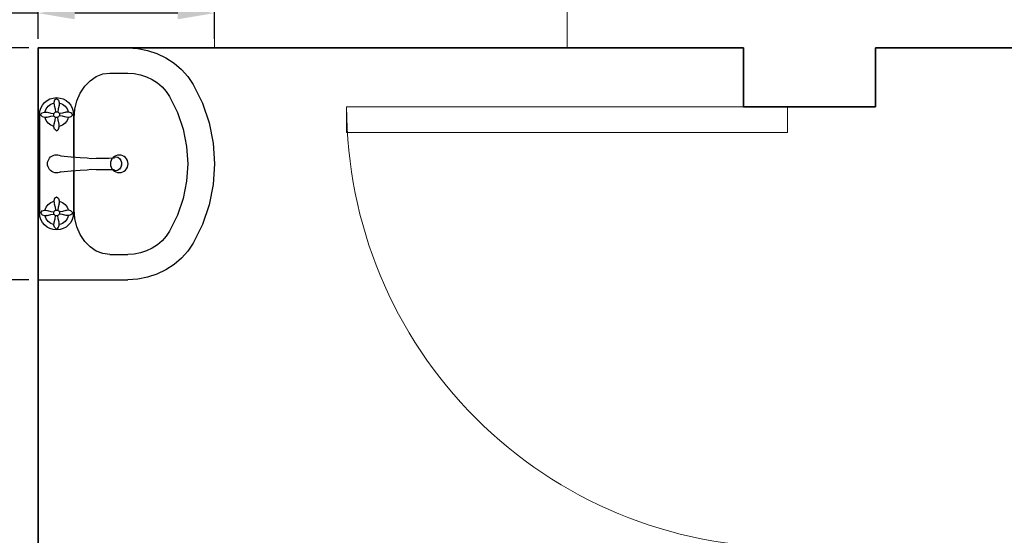
# Model space of a CAD drawing. Units: inches. Extents: x 3321 to 5237, y 11 to 1752.
# Tile 41 of 43: x 4943 to 5010, y 1645 to 1680. Entities that reach past the tile are written whole.
import ezdxf

# ---------------------------------------------------------------- set-up
doc = ezdxf.new("R2010")
doc.units = ezdxf.units.IN
for name, color, linetype, lineweight in [('A-ANNO-DIMS', 2, 'Continuous', 18), ('A-DOOR', 4, 'Continuous', 18), ('A-GLAZ', 5, 'Continuous', 18), ('A-WALL', 7, 'Continuous', 35), ('Сантехника', 7, 'Continuous', 18)]:
    doc.layers.add(name, color=color, linetype=linetype, lineweight=lineweight)
doc.layers.add('SANTEH', color=7, linetype='Continuous')
doc.styles.get("Standard").update_dxf_attribs({"font": 'arial.ttf'})
doc.dimstyles.new('ISO-25', dxfattribs={"dimtxt": 9, "dimasz": 2.5, "dimexe": 1.25, "dimexo": 0.625, "dimtad": 1, "dimdec": 1, "dimlunit": 3, "dimtxsty": 'Standard', "dimcen": 2.5, "dimclrd": 4, "dimclre": 4, "dimclrt": 256, "dimadec": 0, "dimazin": 0, "dimtfac": 1, "dimtdec": 1, "dimtmove": 0, "dimatfit": 3, "dimfxl": 1, "dimarcsym": 0})

# ---------------------------------------------------------------- blocks, each defined once
blk = doc.blocks.new('*U7')
for p, q in [((0, 0), (0, 6)), ((30, 0), (30, 6))]:
    blk.add_line(p, q)
blk.add_lwpolyline([(0, 0), (0, -30), (1.75, -30), (1.75, 0)], close=True)
blk.add_arc((0, 0), 30, 270, 0)
blk = doc.blocks.new('Basin 01_71')
at = {"layer": 'SANTEH'}
for p, q in [((0, 350), (0, 171.8)), ((460, 350), (0, 350)), ((128.5, 341.7), (127.2, 337.2)), ((128.5, 341.7), (127.2, 337.2)), ((128.5, 341.7), (127.2, 337.2)), ((128.5, 341.7), (127.2, 337.2)), ((128.5, 341.7), (127.2, 337.2)), ((128.5, 341.7), (127.2, 337.2)), ((127.2, 337.2), (127.5, 332.3)), ((127.2, 337.2), (127.5, 332.3)), ((127.2, 337.2), (127.5, 332.3)), ((127.2, 337.2), (127.5, 332.3)), ((127.2, 337.2), (127.5, 332.3)), ((127.2, 337.2), (127.5, 332.3)), ((127.5, 332.3), (128.4, 332)), ((127.5, 332.3), (128.4, 332)), ((127.5, 332.3), (128.4, 332)), ((127.5, 332.3), (128.4, 332)), ((127.5, 332.3), (128.4, 332)), ((127.5, 332.3), (128.4, 332)), ((130.2, 343.2), (128.5, 341.7)), ((130.2, 343.2), (128.5, 341.7)), ((130.2, 343.2), (128.5, 341.7)), ((130.2, 343.2), (128.5, 341.7)), ((130.2, 343.2), (128.5, 341.7)), ((130.2, 343.2), (128.5, 341.7)), ((132.5, 345.3), (130.2, 343.2)), ((132.5, 345.3), (130.2, 343.2)), ((132.5, 345.3), (130.2, 343.2)), ((132.5, 345.3), (130.2, 343.2)), ((132.5, 345.3), (130.2, 343.2)), ((132.5, 345.3), (130.2, 343.2)), ((132.5, 346.9), (327.5, 346.9)), ((132.5, 345.3), (134.7, 343.2)), ((132.5, 345.3), (134.7, 343.2)), ((132.5, 345.3), (134.7, 343.2)), ((132.5, 345.3), (134.7, 343.2)), ((132.5, 345.3), (134.7, 343.2)), ((132.5, 345.3), (134.7, 343.2)), ((134.7, 343.2), (136.4, 341.7)), ((134.7, 343.2), (136.4, 341.7)), ((134.7, 343.2), (136.4, 341.7)), ((134.7, 343.2), (136.4, 341.7)), ((134.7, 343.2), (136.4, 341.7)), ((134.7, 343.2), (136.4, 341.7)), ((136.4, 341.7), (137.7, 337.2)), ((136.4, 341.7), (137.7, 337.2)), ((136.4, 341.7), (137.7, 337.2)), ((136.4, 341.7), (137.7, 337.2)), ((136.4, 341.7), (137.7, 337.2)), ((136.4, 341.7), (137.7, 337.2)), ((137.4, 332.3), (136.6, 332)), ((137.4, 332.3), (136.6, 332)), ((137.4, 332.3), (136.6, 332)), ((137.4, 332.3), (136.6, 332)), ((137.4, 332.3), (136.6, 332)), ((137.4, 332.3), (136.6, 332)), ((137.7, 337.2), (137.4, 332.3)), ((137.7, 337.2), (137.4, 332.3)), ((137.7, 337.2), (137.4, 332.3)), ((137.7, 337.2), (137.4, 332.3)), ((137.7, 337.2), (137.4, 332.3)), ((137.7, 337.2), (137.4, 332.3)), ((323.5, 341.7), (322.2, 337.2)), ((323.5, 341.7), (322.2, 337.2)), ((323.5, 341.7), (322.2, 337.2)), ((323.5, 341.7), (322.2, 337.2)), ((323.5, 341.7), (322.2, 337.2)), ((323.5, 341.7), (322.2, 337.2)), ((322.2, 337.2), (322.5, 332.3)), ((322.2, 337.2), (322.5, 332.3)), ((322.2, 337.2), (322.5, 332.3)), ((322.2, 337.2), (322.5, 332.3)), ((322.2, 337.2), (322.5, 332.3)), ((322.2, 337.2), (322.5, 332.3)), ((322.5, 332.3), (323.4, 332)), ((322.5, 332.3), (323.4, 332)), ((322.5, 332.3), (323.4, 332)), ((322.5, 332.3), (323.4, 332)), ((322.5, 332.3), (323.4, 332)), ((322.5, 332.3), (323.4, 332)), ((325.2, 343.2), (323.5, 341.7)), ((325.2, 343.2), (323.5, 341.7)), ((325.2, 343.2), (323.5, 341.7)), ((325.2, 343.2), (323.5, 341.7)), ((325.2, 343.2), (323.5, 341.7)), ((325.2, 343.2), (323.5, 341.7)), ((327.5, 345.3), (325.2, 343.2)), ((327.5, 345.3), (325.2, 343.2)), ((327.5, 345.3), (325.2, 343.2)), ((327.5, 345.3), (325.2, 343.2)), ((327.5, 345.3), (325.2, 343.2)), ((327.5, 345.3), (325.2, 343.2)), ((327.5, 345.3), (329.7, 343.2)), ((327.5, 345.3), (329.7, 343.2)), ((327.5, 345.3), (329.7, 343.2)), ((327.5, 345.3), (329.7, 343.2)), ((327.5, 345.3), (329.7, 343.2)), ((327.5, 345.3), (329.7, 343.2)), ((329.7, 343.2), (331.4, 341.7)), ((329.7, 343.2), (331.4, 341.7)), ((329.7, 343.2), (331.4, 341.7)), ((329.7, 343.2), (331.4, 341.7)), ((329.7, 343.2), (331.4, 341.7)), ((329.7, 343.2), (331.4, 341.7)), ((331.4, 341.7), (332.7, 337.2)), ((331.4, 341.7), (332.7, 337.2)), ((331.4, 341.7), (332.7, 337.2)), ((331.4, 341.7), (332.7, 337.2)), ((331.4, 341.7), (332.7, 337.2)), ((331.4, 341.7), (332.7, 337.2)), ((332.4, 332.3), (331.6, 332)), ((332.4, 332.3), (331.6, 332)), ((332.4, 332.3), (331.6, 332)), ((332.4, 332.3), (331.6, 332)), ((332.4, 332.3), (331.6, 332)), ((332.4, 332.3), (331.6, 332)), ((332.7, 337.2), (332.4, 332.3)), ((332.7, 337.2), (332.4, 332.3)), ((332.7, 337.2), (332.4, 332.3)), ((332.7, 337.2), (332.4, 332.3)), ((332.7, 337.2), (332.4, 332.3)), ((332.7, 337.2), (332.4, 332.3)), ((460, 350), (460, 171.8)), ((100.4, 313.2), (102.5, 315.4)), ((100.4, 313.2), (102.5, 315.4)), ((100.4, 313.2), (102.5, 315.4)), ((100.4, 313.2), (102.5, 315.4)), ((100.4, 313.2), (102.5, 315.4)), ((100.4, 313.2), (102.5, 315.4)), ((100.4, 313.2), (102.5, 310.9)), ((100.4, 313.2), (102.5, 310.9)), ((100.4, 313.2), (102.5, 310.9)), ((100.4, 313.2), (102.5, 310.9)), ((100.4, 313.2), (102.5, 310.9)), ((100.4, 313.2), (102.5, 310.9)), ((102.5, 315.4), (104, 317.1)), ((102.5, 315.4), (104, 317.1)), ((102.5, 315.4), (104, 317.1)), ((102.5, 315.4), (104, 317.1)), ((102.5, 315.4), (104, 317.1)), ((102.5, 315.4), (104, 317.1)), ((104, 317.1), (108.5, 318.4)), ((104, 317.1), (108.5, 318.4)), ((104, 317.1), (108.5, 318.4)), ((104, 317.1), (108.5, 318.4)), ((104, 317.1), (108.5, 318.4)), ((104, 317.1), (108.5, 318.4)), ((108.5, 318.4), (113.4, 318.1)), ((108.5, 318.4), (113.4, 318.1)), ((108.5, 318.4), (113.4, 318.1)), ((108.5, 318.4), (113.4, 318.1)), ((108.5, 318.4), (113.4, 318.1)), ((108.5, 318.4), (113.4, 318.1)), ((113.4, 318.1), (113.7, 317.3)), ((113.4, 318.1), (113.7, 317.3)), ((113.4, 318.1), (113.7, 317.3)), ((113.4, 318.1), (113.7, 317.3)), ((113.4, 318.1), (113.7, 317.3)), ((113.4, 318.1), (113.7, 317.3)), ((113.7, 317.3), (114.2, 318.1)), ((113.7, 317.3), (114.2, 318.1)), ((113.7, 317.3), (114.2, 318.1)), ((113.7, 317.3), (114.2, 318.1)), ((113.7, 317.3), (114.2, 318.1)), ((113.7, 317.3), (114.2, 318.1)), ((114.2, 318.1), (121, 316.1)), ((114.2, 318.1), (121, 316.1)), ((114.2, 318.1), (121, 316.1)), ((114.2, 318.1), (121, 316.1)), ((114.2, 318.1), (121, 316.1)), ((114.2, 318.1), (121, 316.1)), ((121, 316.1), (127.3, 315.5)), ((121, 316.1), (127.3, 315.5)), ((121, 316.1), (127.3, 315.5)), ((121, 316.1), (127.3, 315.5)), ((121, 316.1), (127.3, 315.5)), ((121, 316.1), (127.3, 315.5)), ((127.1, 315.1), (126.8, 313.9)), ((127.1, 315.1), (126.8, 313.9)), ((127.1, 315.1), (126.8, 313.9)), ((127.1, 315.1), (126.8, 313.9)), ((127.1, 315.1), (126.8, 313.9)), ((127.1, 315.1), (126.8, 313.9)), ((126.8, 313.9), (126.8, 312.5)), ((126.8, 313.9), (126.8, 312.5)), ((126.8, 313.9), (126.8, 312.5)), ((126.8, 313.9), (126.8, 312.5)), ((126.8, 313.9), (126.8, 312.5)), ((126.8, 313.9), (126.8, 312.5)), ((126.8, 312.5), (127.1, 311.2)), ((126.8, 312.5), (127.1, 311.2)), ((126.8, 312.5), (127.1, 311.2)), ((126.8, 312.5), (127.1, 311.2)), ((126.8, 312.5), (127.1, 311.2)), ((126.8, 312.5), (127.1, 311.2)), ((127.7, 316.3), (127.1, 315.1)), ((127.7, 316.3), (127.1, 315.1)), ((127.7, 316.3), (127.1, 315.1)), ((127.7, 316.3), (127.1, 315.1)), ((127.7, 316.3), (127.1, 315.1)), ((127.7, 316.3), (127.1, 315.1)), ((128.4, 332), (127.6, 331.5)), ((128.4, 332), (127.6, 331.5)), ((128.4, 332), (127.6, 331.5)), ((128.4, 332), (127.6, 331.5)), ((128.4, 332), (127.6, 331.5)), ((128.4, 332), (127.6, 331.5)), ((127.6, 331.5), (129.6, 324.7)), ((127.6, 331.5), (129.6, 324.7)), ((127.6, 331.5), (129.6, 324.7)), ((127.6, 331.5), (129.6, 324.7)), ((127.6, 331.5), (129.6, 324.7)), ((127.6, 331.5), (129.6, 324.7)), ((128.6, 317.3), (127.7, 316.3)), ((128.6, 317.3), (127.7, 316.3)), ((128.6, 317.3), (127.7, 316.3)), ((128.6, 317.3), (127.7, 316.3)), ((128.6, 317.3), (127.7, 316.3)), ((128.6, 317.3), (127.7, 316.3)), ((129.7, 318.1), (128.6, 317.3)), ((129.7, 318.1), (128.6, 317.3)), ((129.7, 318.1), (128.6, 317.3)), ((129.7, 318.1), (128.6, 317.3)), ((129.7, 318.1), (128.6, 317.3)), ((129.7, 318.1), (128.6, 317.3)), ((129.6, 324.7), (130.2, 318.4)), ((129.6, 324.7), (130.2, 318.4)), ((129.6, 324.7), (130.2, 318.4)), ((129.6, 324.7), (130.2, 318.4)), ((129.6, 324.7), (130.2, 318.4)), ((129.6, 324.7), (130.2, 318.4)), ((130.9, 318.7), (129.7, 318.1)), ((130.9, 318.7), (129.7, 318.1)), ((130.9, 318.7), (129.7, 318.1)), ((130.9, 318.7), (129.7, 318.1)), ((130.9, 318.7), (129.7, 318.1)), ((130.9, 318.7), (129.7, 318.1)), ((132.2, 318.9), (130.9, 318.7)), ((132.2, 318.9), (130.9, 318.7)), ((132.2, 318.9), (130.9, 318.7)), ((132.2, 318.9), (130.9, 318.7)), ((132.2, 318.9), (130.9, 318.7)), ((132.2, 318.9), (130.9, 318.7)), ((133.5, 318.8), (132.2, 318.9)), ((133.5, 318.8), (132.2, 318.9)), ((133.5, 318.8), (132.2, 318.9)), ((133.5, 318.8), (132.2, 318.9)), ((133.5, 318.8), (132.2, 318.9)), ((133.5, 318.8), (132.2, 318.9)), ((134.8, 318.4), (133.5, 318.8)), ((134.8, 318.4), (133.5, 318.8)), ((134.8, 318.4), (133.5, 318.8)), ((134.8, 318.4), (133.5, 318.8)), ((134.8, 318.4), (133.5, 318.8)), ((134.8, 318.4), (133.5, 318.8)), ((135.4, 324.7), (134.8, 318.4)), ((135.4, 324.7), (134.8, 318.4)), ((135.4, 324.7), (134.8, 318.4)), ((135.4, 324.7), (134.8, 318.4)), ((135.4, 324.7), (134.8, 318.4)), ((135.4, 324.7), (134.8, 318.4)), ((135.9, 317.8), (134.8, 318.4)), ((135.9, 317.8), (134.8, 318.4)), ((135.9, 317.8), (134.8, 318.4)), ((135.9, 317.8), (134.8, 318.4)), ((135.9, 317.8), (134.8, 318.4)), ((135.9, 317.8), (134.8, 318.4)), ((137.4, 331.5), (135.4, 324.7)), ((137.4, 331.5), (135.4, 324.7)), ((137.4, 331.5), (135.4, 324.7)), ((137.4, 331.5), (135.4, 324.7)), ((137.4, 331.5), (135.4, 324.7)), ((137.4, 331.5), (135.4, 324.7)), ((136.9, 316.9), (135.9, 317.8)), ((136.9, 316.9), (135.9, 317.8)), ((136.9, 316.9), (135.9, 317.8)), ((136.9, 316.9), (135.9, 317.8)), ((136.9, 316.9), (135.9, 317.8)), ((136.9, 316.9), (135.9, 317.8)), ((136.6, 332), (137.4, 331.5)), ((136.6, 332), (137.4, 331.5)), ((136.6, 332), (137.4, 331.5)), ((136.6, 332), (137.4, 331.5)), ((136.6, 332), (137.4, 331.5)), ((136.6, 332), (137.4, 331.5)), ((137.6, 315.8), (136.9, 316.9)), ((137.6, 315.8), (136.9, 316.9)), ((137.6, 315.8), (136.9, 316.9)), ((137.6, 315.8), (136.9, 316.9)), ((137.6, 315.8), (136.9, 316.9)), ((137.6, 315.8), (136.9, 316.9)), ((138, 314.5), (137.6, 315.8)), ((138, 314.5), (137.6, 315.8)), ((138, 314.5), (137.6, 315.8)), ((138, 314.5), (137.6, 315.8)), ((138, 314.5), (137.6, 315.8)), ((138, 314.5), (137.6, 315.8)), ((144, 316.1), (137.7, 315.5)), ((144, 316.1), (137.7, 315.5)), ((144, 316.1), (137.7, 315.5)), ((144, 316.1), (137.7, 315.5)), ((144, 316.1), (137.7, 315.5)), ((144, 316.1), (137.7, 315.5)), ((138.2, 313.2), (138, 314.5)), ((138.2, 313.2), (138, 314.5)), ((138.2, 313.2), (138, 314.5)), ((138.2, 313.2), (138, 314.5)), ((138.2, 313.2), (138, 314.5)), ((138.2, 313.2), (138, 314.5)), ((138, 311.9), (138.2, 313.2)), ((138, 311.9), (138.2, 313.2)), ((138, 311.9), (138.2, 313.2)), ((138, 311.9), (138.2, 313.2)), ((138, 311.9), (138.2, 313.2)), ((138, 311.9), (138.2, 313.2)), ((150.8, 318.1), (144, 316.1)), ((150.8, 318.1), (144, 316.1)), ((150.8, 318.1), (144, 316.1)), ((150.8, 318.1), (144, 316.1)), ((150.8, 318.1), (144, 316.1)), ((150.8, 318.1), (144, 316.1)), ((151.3, 317.3), (150.8, 318.1)), ((151.3, 317.3), (150.8, 318.1)), ((151.3, 317.3), (150.8, 318.1)), ((151.3, 317.3), (150.8, 318.1)), ((151.3, 317.3), (150.8, 318.1)), ((151.3, 317.3), (150.8, 318.1)), ((151.6, 318.1), (151.3, 317.3)), ((151.6, 318.1), (151.3, 317.3)), ((151.6, 318.1), (151.3, 317.3)), ((151.6, 318.1), (151.3, 317.3)), ((151.6, 318.1), (151.3, 317.3)), ((151.6, 318.1), (151.3, 317.3)), ((156.5, 318.4), (151.6, 318.1)), ((156.5, 318.4), (151.6, 318.1)), ((156.5, 318.4), (151.6, 318.1)), ((156.5, 318.4), (151.6, 318.1)), ((156.5, 318.4), (151.6, 318.1)), ((156.5, 318.4), (151.6, 318.1)), ((161, 317.2), (156.5, 318.4)), ((161, 317.2), (156.5, 318.4)), ((161, 317.2), (156.5, 318.4)), ((161, 317.2), (156.5, 318.4)), ((161, 317.2), (156.5, 318.4)), ((161, 317.2), (156.5, 318.4)), ((162.5, 315.4), (161, 317.2)), ((162.5, 315.4), (161, 317.2)), ((162.5, 315.4), (161, 317.2)), ((162.5, 315.4), (161, 317.2)), ((162.5, 315.4), (161, 317.2)), ((162.5, 315.4), (161, 317.2)), ((164.6, 313.2), (162.5, 315.4)), ((164.6, 313.2), (162.5, 315.4)), ((164.6, 313.2), (162.5, 315.4)), ((164.6, 313.2), (162.5, 315.4)), ((164.6, 313.2), (162.5, 315.4)), ((164.6, 313.2), (162.5, 315.4)), ((164.6, 313.2), (162.5, 311)), ((164.6, 313.2), (162.5, 311)), ((164.6, 313.2), (162.5, 311)), ((164.6, 313.2), (162.5, 311)), ((164.6, 313.2), (162.5, 311)), ((164.6, 313.2), (162.5, 311)), ((295.4, 313.2), (297.5, 315.4)), ((295.4, 313.2), (297.5, 315.4)), ((295.4, 313.2), (297.5, 315.4)), ((295.4, 313.2), (297.5, 315.4)), ((295.4, 313.2), (297.5, 315.4)), ((295.4, 313.2), (297.5, 315.4)), ((295.4, 313.2), (297.5, 310.9)), ((295.4, 313.2), (297.5, 310.9)), ((295.4, 313.2), (297.5, 310.9)), ((295.4, 313.2), (297.5, 310.9)), ((295.4, 313.2), (297.5, 310.9)), ((295.4, 313.2), (297.5, 310.9)), ((297.5, 315.4), (299, 317.1)), ((297.5, 315.4), (299, 317.1)), ((297.5, 315.4), (299, 317.1)), ((297.5, 315.4), (299, 317.1)), ((297.5, 315.4), (299, 317.1)), ((297.5, 315.4), (299, 317.1)), ((299, 317.1), (303.5, 318.4)), ((299, 317.1), (303.5, 318.4)), ((299, 317.1), (303.5, 318.4)), ((299, 317.1), (303.5, 318.4)), ((299, 317.1), (303.5, 318.4)), ((299, 317.1), (303.5, 318.4)), ((303.5, 318.4), (308.4, 318.1)), ((303.5, 318.4), (308.4, 318.1)), ((303.5, 318.4), (308.4, 318.1)), ((303.5, 318.4), (308.4, 318.1)), ((303.5, 318.4), (308.4, 318.1)), ((303.5, 318.4), (308.4, 318.1)), ((308.4, 318.1), (308.7, 317.3)), ((308.4, 318.1), (308.7, 317.3)), ((308.4, 318.1), (308.7, 317.3)), ((308.4, 318.1), (308.7, 317.3)), ((308.4, 318.1), (308.7, 317.3)), ((308.4, 318.1), (308.7, 317.3)), ((308.7, 317.3), (309.2, 318.1)), ((308.7, 317.3), (309.2, 318.1)), ((308.7, 317.3), (309.2, 318.1)), ((308.7, 317.3), (309.2, 318.1)), ((308.7, 317.3), (309.2, 318.1)), ((308.7, 317.3), (309.2, 318.1)), ((309.2, 318.1), (316, 316.1)), ((309.2, 318.1), (316, 316.1)), ((309.2, 318.1), (316, 316.1)), ((309.2, 318.1), (316, 316.1)), ((309.2, 318.1), (316, 316.1)), ((309.2, 318.1), (316, 316.1)), ((316, 316.1), (322.3, 315.5)), ((316, 316.1), (322.3, 315.5)), ((316, 316.1), (322.3, 315.5)), ((316, 316.1), (322.3, 315.5)), ((316, 316.1), (322.3, 315.5)), ((316, 316.1), (322.3, 315.5)), ((322.1, 315.1), (321.8, 313.9)), ((322.1, 315.1), (321.8, 313.9)), ((322.1, 315.1), (321.8, 313.9)), ((322.1, 315.1), (321.8, 313.9)), ((322.1, 315.1), (321.8, 313.9)), ((322.1, 315.1), (321.8, 313.9)), ((321.8, 313.9), (321.8, 312.5)), ((321.8, 313.9), (321.8, 312.5)), ((321.8, 313.9), (321.8, 312.5)), ((321.8, 313.9), (321.8, 312.5)), ((321.8, 313.9), (321.8, 312.5)), ((321.8, 313.9), (321.8, 312.5)), ((321.8, 312.5), (322.1, 311.2)), ((321.8, 312.5), (322.1, 311.2)), ((321.8, 312.5), (322.1, 311.2)), ((321.8, 312.5), (322.1, 311.2)), ((321.8, 312.5), (322.1, 311.2)), ((321.8, 312.5), (322.1, 311.2)), ((322.7, 316.3), (322.1, 315.1)), ((322.7, 316.3), (322.1, 315.1)), ((322.7, 316.3), (322.1, 315.1)), ((322.7, 316.3), (322.1, 315.1)), ((322.7, 316.3), (322.1, 315.1)), ((322.7, 316.3), (322.1, 315.1)), ((323.4, 332), (322.6, 331.5)), ((323.4, 332), (322.6, 331.5)), ((323.4, 332), (322.6, 331.5)), ((323.4, 332), (322.6, 331.5)), ((323.4, 332), (322.6, 331.5)), ((323.4, 332), (322.6, 331.5)), ((322.6, 331.5), (324.6, 324.7)), ((322.6, 331.5), (324.6, 324.7)), ((322.6, 331.5), (324.6, 324.7)), ((322.6, 331.5), (324.6, 324.7)), ((322.6, 331.5), (324.6, 324.7)), ((322.6, 331.5), (324.6, 324.7)), ((323.6, 317.3), (322.7, 316.3)), ((323.6, 317.3), (322.7, 316.3)), ((323.6, 317.3), (322.7, 316.3)), ((323.6, 317.3), (322.7, 316.3)), ((323.6, 317.3), (322.7, 316.3)), ((323.6, 317.3), (322.7, 316.3)), ((324.7, 318.1), (323.6, 317.3)), ((324.7, 318.1), (323.6, 317.3)), ((324.7, 318.1), (323.6, 317.3)), ((324.7, 318.1), (323.6, 317.3)), ((324.7, 318.1), (323.6, 317.3)), ((324.7, 318.1), (323.6, 317.3)), ((324.6, 324.7), (325.2, 318.4)), ((324.6, 324.7), (325.2, 318.4)), ((324.6, 324.7), (325.2, 318.4)), ((324.6, 324.7), (325.2, 318.4)), ((324.6, 324.7), (325.2, 318.4)), ((324.6, 324.7), (325.2, 318.4)), ((325.9, 318.7), (324.7, 318.1)), ((325.9, 318.7), (324.7, 318.1)), ((325.9, 318.7), (324.7, 318.1)), ((325.9, 318.7), (324.7, 318.1)), ((325.9, 318.7), (324.7, 318.1)), ((325.9, 318.7), (324.7, 318.1)), ((327.2, 318.9), (325.9, 318.7)), ((327.2, 318.9), (325.9, 318.7)), ((327.2, 318.9), (325.9, 318.7)), ((327.2, 318.9), (325.9, 318.7)), ((327.2, 318.9), (325.9, 318.7)), ((327.2, 318.9), (325.9, 318.7)), ((328.5, 318.8), (327.2, 318.9)), ((328.5, 318.8), (327.2, 318.9)), ((328.5, 318.8), (327.2, 318.9)), ((328.5, 318.8), (327.2, 318.9)), ((328.5, 318.8), (327.2, 318.9)), ((328.5, 318.8), (327.2, 318.9)), ((329.8, 318.4), (328.5, 318.8)), ((329.8, 318.4), (328.5, 318.8)), ((329.8, 318.4), (328.5, 318.8)), ((329.8, 318.4), (328.5, 318.8)), ((329.8, 318.4), (328.5, 318.8)), ((329.8, 318.4), (328.5, 318.8)), ((330.4, 324.7), (329.8, 318.4)), ((330.4, 324.7), (329.8, 318.4)), ((330.4, 324.7), (329.8, 318.4)), ((330.4, 324.7), (329.8, 318.4)), ((330.4, 324.7), (329.8, 318.4)), ((330.4, 324.7), (329.8, 318.4)), ((330.9, 317.8), (329.8, 318.4)), ((330.9, 317.8), (329.8, 318.4)), ((330.9, 317.8), (329.8, 318.4)), ((330.9, 317.8), (329.8, 318.4)), ((330.9, 317.8), (329.8, 318.4)), ((330.9, 317.8), (329.8, 318.4)), ((332.4, 331.5), (330.4, 324.7)), ((332.4, 331.5), (330.4, 324.7)), ((332.4, 331.5), (330.4, 324.7)), ((332.4, 331.5), (330.4, 324.7)), ((332.4, 331.5), (330.4, 324.7)), ((332.4, 331.5), (330.4, 324.7)), ((331.9, 316.9), (330.9, 317.8)), ((331.9, 316.9), (330.9, 317.8)), ((331.9, 316.9), (330.9, 317.8)), ((331.9, 316.9), (330.9, 317.8)), ((331.9, 316.9), (330.9, 317.8)), ((331.9, 316.9), (330.9, 317.8)), ((331.6, 332), (332.4, 331.5)), ((331.6, 332), (332.4, 331.5)), ((331.6, 332), (332.4, 331.5)), ((331.6, 332), (332.4, 331.5)), ((331.6, 332), (332.4, 331.5)), ((331.6, 332), (332.4, 331.5)), ((332.6, 315.8), (331.9, 316.9)), ((332.6, 315.8), (331.9, 316.9)), ((332.6, 315.8), (331.9, 316.9)), ((332.6, 315.8), (331.9, 316.9)), ((332.6, 315.8), (331.9, 316.9)), ((332.6, 315.8), (331.9, 316.9)), ((333, 314.5), (332.6, 315.8)), ((333, 314.5), (332.6, 315.8)), ((333, 314.5), (332.6, 315.8)), ((333, 314.5), (332.6, 315.8)), ((333, 314.5), (332.6, 315.8)), ((333, 314.5), (332.6, 315.8)), ((339, 316.1), (332.7, 315.5)), ((339, 316.1), (332.7, 315.5)), ((339, 316.1), (332.7, 315.5)), ((339, 316.1), (332.7, 315.5)), ((339, 316.1), (332.7, 315.5)), ((339, 316.1), (332.7, 315.5)), ((333.2, 313.2), (333, 314.5)), ((333.2, 313.2), (333, 314.5)), ((333.2, 313.2), (333, 314.5)), ((333.2, 313.2), (333, 314.5)), ((333.2, 313.2), (333, 314.5)), ((333.2, 313.2), (333, 314.5)), ((333, 311.9), (333.2, 313.2)), ((333, 311.9), (333.2, 313.2)), ((333, 311.9), (333.2, 313.2)), ((333, 311.9), (333.2, 313.2)), ((333, 311.9), (333.2, 313.2)), ((333, 311.9), (333.2, 313.2)), ((345.8, 318.1), (339, 316.1)), ((345.8, 318.1), (339, 316.1)), ((345.8, 318.1), (339, 316.1)), ((345.8, 318.1), (339, 316.1)), ((345.8, 318.1), (339, 316.1)), ((345.8, 318.1), (339, 316.1)), ((346.3, 317.3), (345.8, 318.1)), ((346.3, 317.3), (345.8, 318.1)), ((346.3, 317.3), (345.8, 318.1)), ((346.3, 317.3), (345.8, 318.1)), ((346.3, 317.3), (345.8, 318.1)), ((346.3, 317.3), (345.8, 318.1)), ((346.6, 318.1), (346.3, 317.3)), ((346.6, 318.1), (346.3, 317.3)), ((346.6, 318.1), (346.3, 317.3)), ((346.6, 318.1), (346.3, 317.3)), ((346.6, 318.1), (346.3, 317.3)), ((346.6, 318.1), (346.3, 317.3)), ((351.5, 318.4), (346.6, 318.1)), ((351.5, 318.4), (346.6, 318.1)), ((351.5, 318.4), (346.6, 318.1)), ((351.5, 318.4), (346.6, 318.1)), ((351.5, 318.4), (346.6, 318.1)), ((351.5, 318.4), (346.6, 318.1)), ((356, 317.2), (351.5, 318.4)), ((356, 317.2), (351.5, 318.4)), ((356, 317.2), (351.5, 318.4)), ((356, 317.2), (351.5, 318.4)), ((356, 317.2), (351.5, 318.4)), ((356, 317.2), (351.5, 318.4)), ((357.5, 315.4), (356, 317.2)), ((357.5, 315.4), (356, 317.2)), ((357.5, 315.4), (356, 317.2)), ((357.5, 315.4), (356, 317.2)), ((357.5, 315.4), (356, 317.2)), ((357.5, 315.4), (356, 317.2)), ((359.6, 313.2), (357.5, 315.4)), ((359.6, 313.2), (357.5, 315.4)), ((359.6, 313.2), (357.5, 315.4)), ((359.6, 313.2), (357.5, 315.4)), ((359.6, 313.2), (357.5, 315.4)), ((359.6, 313.2), (357.5, 315.4)), ((359.6, 313.2), (357.5, 311)), ((359.6, 313.2), (357.5, 311)), ((359.6, 313.2), (357.5, 311)), ((359.6, 313.2), (357.5, 311)), ((359.6, 313.2), (357.5, 311)), ((359.6, 313.2), (357.5, 311)), ((102.5, 310.9), (104, 309.2)), ((102.5, 310.9), (104, 309.2)), ((102.5, 310.9), (104, 309.2)), ((102.5, 310.9), (104, 309.2)), ((102.5, 310.9), (104, 309.2)), ((102.5, 310.9), (104, 309.2)), ((104, 309.2), (108.5, 307.9)), ((104, 309.2), (108.5, 307.9)), ((104, 309.2), (108.5, 307.9)), ((104, 309.2), (108.5, 307.9)), ((104, 309.2), (108.5, 307.9)), ((104, 309.2), (108.5, 307.9)), ((108.5, 307.9), (113.4, 308.2)), ((108.5, 307.9), (113.4, 308.2)), ((108.5, 307.9), (113.4, 308.2)), ((108.5, 307.9), (113.4, 308.2)), ((108.5, 307.9), (113.4, 308.2)), ((108.5, 307.9), (113.4, 308.2)), ((113.4, 308.2), (113.7, 309.1)), ((113.4, 308.2), (113.7, 309.1)), ((113.4, 308.2), (113.7, 309.1)), ((113.4, 308.2), (113.7, 309.1)), ((113.4, 308.2), (113.7, 309.1)), ((113.4, 308.2), (113.7, 309.1)), ((113.7, 309.1), (114.2, 308.3)), ((113.7, 309.1), (114.2, 308.3)), ((113.7, 309.1), (114.2, 308.3)), ((113.7, 309.1), (114.2, 308.3)), ((113.7, 309.1), (114.2, 308.3)), ((113.7, 309.1), (114.2, 308.3)), ((114.2, 308.3), (121, 310.3)), ((114.2, 308.3), (121, 310.3)), ((114.2, 308.3), (121, 310.3)), ((114.2, 308.3), (121, 310.3)), ((114.2, 308.3), (121, 310.3)), ((114.2, 308.3), (121, 310.3)), ((121, 310.3), (127.3, 310.9)), ((121, 310.3), (127.3, 310.9)), ((121, 310.3), (127.3, 310.9)), ((121, 310.3), (127.3, 310.9)), ((121, 310.3), (127.3, 310.9)), ((121, 310.3), (127.3, 310.9)), ((127.1, 311.2), (127.7, 310.1)), ((127.1, 311.2), (127.7, 310.1)), ((127.1, 311.2), (127.7, 310.1)), ((127.1, 311.2), (127.7, 310.1)), ((127.1, 311.2), (127.7, 310.1)), ((127.1, 311.2), (127.7, 310.1)), ((127.3, 289.2), (127.6, 294.1)), ((127.3, 289.2), (127.6, 294.1)), ((127.3, 289.2), (127.6, 294.1)), ((127.3, 289.2), (127.6, 294.1)), ((127.3, 289.2), (127.6, 294.1)), ((127.3, 289.2), (127.6, 294.1)), ((127.6, 294.9), (129.6, 301.7)), ((127.6, 294.9), (129.6, 301.7)), ((127.6, 294.9), (129.6, 301.7)), ((127.6, 294.9), (129.6, 301.7)), ((127.6, 294.9), (129.6, 301.7)), ((127.6, 294.9), (129.6, 301.7)), ((128.4, 294.4), (127.6, 294.9)), ((128.4, 294.4), (127.6, 294.9)), ((128.4, 294.4), (127.6, 294.9)), ((128.4, 294.4), (127.6, 294.9)), ((128.4, 294.4), (127.6, 294.9)), ((128.4, 294.4), (127.6, 294.9)), ((127.6, 294.1), (128.4, 294.4)), ((127.6, 294.1), (128.4, 294.4)), ((127.6, 294.1), (128.4, 294.4)), ((127.6, 294.1), (128.4, 294.4)), ((127.6, 294.1), (128.4, 294.4)), ((127.6, 294.1), (128.4, 294.4)), ((127.7, 310.1), (128.6, 309.1)), ((127.7, 310.1), (128.6, 309.1)), ((127.7, 310.1), (128.6, 309.1)), ((127.7, 310.1), (128.6, 309.1)), ((127.7, 310.1), (128.6, 309.1)), ((127.7, 310.1), (128.6, 309.1)), ((128.6, 309.1), (129.7, 308.3)), ((128.6, 309.1), (129.7, 308.3)), ((128.6, 309.1), (129.7, 308.3)), ((128.6, 309.1), (129.7, 308.3)), ((128.6, 309.1), (129.7, 308.3)), ((128.6, 309.1), (129.7, 308.3)), ((129.6, 301.7), (130.2, 308)), ((129.6, 301.7), (130.2, 308)), ((129.6, 301.7), (130.2, 308)), ((129.6, 301.7), (130.2, 308)), ((129.6, 301.7), (130.2, 308)), ((129.6, 301.7), (130.2, 308)), ((129.7, 308.3), (130.9, 307.7)), ((129.7, 308.3), (130.9, 307.7)), ((129.7, 308.3), (130.9, 307.7)), ((129.7, 308.3), (130.9, 307.7)), ((129.7, 308.3), (130.9, 307.7)), ((129.7, 308.3), (130.9, 307.7)), ((130.9, 307.7), (132.2, 307.5)), ((130.9, 307.7), (132.2, 307.5)), ((130.9, 307.7), (132.2, 307.5)), ((130.9, 307.7), (132.2, 307.5)), ((130.9, 307.7), (132.2, 307.5)), ((130.9, 307.7), (132.2, 307.5)), ((132.2, 307.5), (133.5, 307.6)), ((132.2, 307.5), (133.5, 307.6)), ((132.2, 307.5), (133.5, 307.6)), ((132.2, 307.5), (133.5, 307.6)), ((132.2, 307.5), (133.5, 307.6)), ((132.2, 307.5), (133.5, 307.6)), ((133.5, 307.6), (134.8, 308)), ((133.5, 307.6), (134.8, 308)), ((133.5, 307.6), (134.8, 308)), ((133.5, 307.6), (134.8, 308)), ((133.5, 307.6), (134.8, 308)), ((133.5, 307.6), (134.8, 308)), ((134.8, 308), (135.9, 308.6)), ((134.8, 308), (135.9, 308.6)), ((134.8, 308), (135.9, 308.6)), ((134.8, 308), (135.9, 308.6)), ((134.8, 308), (135.9, 308.6)), ((134.8, 308), (135.9, 308.6)), ((135.4, 301.7), (134.8, 308)), ((135.4, 301.7), (134.8, 308)), ((135.4, 301.7), (134.8, 308)), ((135.4, 301.7), (134.8, 308)), ((135.4, 301.7), (134.8, 308)), ((135.4, 301.7), (134.8, 308)), ((137.4, 294.9), (135.4, 301.7)), ((137.4, 294.9), (135.4, 301.7)), ((137.4, 294.9), (135.4, 301.7)), ((137.4, 294.9), (135.4, 301.7)), ((137.4, 294.9), (135.4, 301.7)), ((137.4, 294.9), (135.4, 301.7)), ((135.9, 308.6), (136.9, 309.5)), ((135.9, 308.6), (136.9, 309.5)), ((135.9, 308.6), (136.9, 309.5)), ((135.9, 308.6), (136.9, 309.5)), ((135.9, 308.6), (136.9, 309.5)), ((135.9, 308.6), (136.9, 309.5)), ((136.6, 294.4), (137.4, 294.9)), ((136.6, 294.4), (137.4, 294.9)), ((136.6, 294.4), (137.4, 294.9)), ((136.6, 294.4), (137.4, 294.9)), ((136.6, 294.4), (137.4, 294.9)), ((136.6, 294.4), (137.4, 294.9)), ((137.5, 294.1), (136.6, 294.4)), ((137.5, 294.1), (136.6, 294.4)), ((137.5, 294.1), (136.6, 294.4)), ((137.5, 294.1), (136.6, 294.4)), ((137.5, 294.1), (136.6, 294.4)), ((137.5, 294.1), (136.6, 294.4)), ((136.9, 309.5), (137.6, 310.6)), ((136.9, 309.5), (137.6, 310.6)), ((136.9, 309.5), (137.6, 310.6)), ((136.9, 309.5), (137.6, 310.6)), ((136.9, 309.5), (137.6, 310.6)), ((136.9, 309.5), (137.6, 310.6)), ((137.8, 289.2), (137.5, 294.1)), ((137.8, 289.2), (137.5, 294.1)), ((137.8, 289.2), (137.5, 294.1)), ((137.8, 289.2), (137.5, 294.1)), ((137.8, 289.2), (137.5, 294.1)), ((137.8, 289.2), (137.5, 294.1)), ((137.6, 310.6), (138, 311.9)), ((137.6, 310.6), (138, 311.9)), ((137.6, 310.6), (138, 311.9)), ((137.6, 310.6), (138, 311.9)), ((137.6, 310.6), (138, 311.9)), ((137.6, 310.6), (138, 311.9)), ((144, 310.3), (137.7, 310.9)), ((144, 310.3), (137.7, 310.9)), ((144, 310.3), (137.7, 310.9)), ((144, 310.3), (137.7, 310.9)), ((144, 310.3), (137.7, 310.9)), ((144, 310.3), (137.7, 310.9)), ((150.8, 308.3), (144, 310.3)), ((150.8, 308.3), (144, 310.3)), ((150.8, 308.3), (144, 310.3)), ((150.8, 308.3), (144, 310.3)), ((150.8, 308.3), (144, 310.3)), ((150.8, 308.3), (144, 310.3)), ((151.3, 309.1), (150.8, 308.3)), ((151.3, 309.1), (150.8, 308.3)), ((151.3, 309.1), (150.8, 308.3)), ((151.3, 309.1), (150.8, 308.3)), ((151.3, 309.1), (150.8, 308.3)), ((151.3, 309.1), (150.8, 308.3)), ((151.6, 308.3), (151.3, 309.1)), ((151.6, 308.3), (151.3, 309.1)), ((151.6, 308.3), (151.3, 309.1)), ((151.6, 308.3), (151.3, 309.1)), ((151.6, 308.3), (151.3, 309.1)), ((151.6, 308.3), (151.3, 309.1)), ((156.5, 308), (151.6, 308.3)), ((156.5, 308), (151.6, 308.3)), ((156.5, 308), (151.6, 308.3)), ((156.5, 308), (151.6, 308.3)), ((156.5, 308), (151.6, 308.3)), ((156.5, 308), (151.6, 308.3)), ((161, 309.2), (156.5, 308)), ((161, 309.2), (156.5, 308)), ((161, 309.2), (156.5, 308)), ((161, 309.2), (156.5, 308)), ((161, 309.2), (156.5, 308)), ((161, 309.2), (156.5, 308)), ((162.5, 311), (161, 309.2)), ((162.5, 311), (161, 309.2)), ((162.5, 311), (161, 309.2)), ((162.5, 311), (161, 309.2)), ((162.5, 311), (161, 309.2)), ((162.5, 311), (161, 309.2)), ((213.9, 305.1), (215, 298)), ((215, 298), (216.2, 284.6)), ((245, 298), (243.8, 284.6)), ((246.1, 305.1), (245, 298)), ((297.5, 310.9), (299, 309.2)), ((297.5, 310.9), (299, 309.2)), ((297.5, 310.9), (299, 309.2)), ((297.5, 310.9), (299, 309.2)), ((297.5, 310.9), (299, 309.2)), ((297.5, 310.9), (299, 309.2)), ((299, 309.2), (303.5, 307.9)), ((299, 309.2), (303.5, 307.9)), ((299, 309.2), (303.5, 307.9)), ((299, 309.2), (303.5, 307.9)), ((299, 309.2), (303.5, 307.9)), ((299, 309.2), (303.5, 307.9)), ((303.5, 307.9), (308.4, 308.2)), ((303.5, 307.9), (308.4, 308.2)), ((303.5, 307.9), (308.4, 308.2)), ((303.5, 307.9), (308.4, 308.2)), ((303.5, 307.9), (308.4, 308.2)), ((303.5, 307.9), (308.4, 308.2)), ((308.4, 308.2), (308.7, 309.1)), ((308.4, 308.2), (308.7, 309.1)), ((308.4, 308.2), (308.7, 309.1)), ((308.4, 308.2), (308.7, 309.1)), ((308.4, 308.2), (308.7, 309.1)), ((308.4, 308.2), (308.7, 309.1)), ((308.7, 309.1), (309.2, 308.3)), ((308.7, 309.1), (309.2, 308.3)), ((308.7, 309.1), (309.2, 308.3)), ((308.7, 309.1), (309.2, 308.3)), ((308.7, 309.1), (309.2, 308.3)), ((308.7, 309.1), (309.2, 308.3)), ((309.2, 308.3), (316, 310.3)), ((309.2, 308.3), (316, 310.3)), ((309.2, 308.3), (316, 310.3)), ((309.2, 308.3), (316, 310.3)), ((309.2, 308.3), (316, 310.3)), ((309.2, 308.3), (316, 310.3)), ((316, 310.3), (322.3, 310.9)), ((316, 310.3), (322.3, 310.9)), ((316, 310.3), (322.3, 310.9)), ((316, 310.3), (322.3, 310.9)), ((316, 310.3), (322.3, 310.9)), ((316, 310.3), (322.3, 310.9)), ((322.1, 311.2), (322.7, 310.1)), ((322.1, 311.2), (322.7, 310.1)), ((322.1, 311.2), (322.7, 310.1)), ((322.1, 311.2), (322.7, 310.1)), ((322.1, 311.2), (322.7, 310.1)), ((322.1, 311.2), (322.7, 310.1)), ((322.3, 289.2), (322.6, 294.1)), ((322.3, 289.2), (322.6, 294.1)), ((322.3, 289.2), (322.6, 294.1)), ((322.3, 289.2), (322.6, 294.1)), ((322.3, 289.2), (322.6, 294.1)), ((322.3, 289.2), (322.6, 294.1)), ((322.6, 294.9), (324.6, 301.7)), ((322.6, 294.9), (324.6, 301.7)), ((322.6, 294.9), (324.6, 301.7)), ((322.6, 294.9), (324.6, 301.7)), ((322.6, 294.9), (324.6, 301.7)), ((322.6, 294.9), (324.6, 301.7)), ((323.4, 294.4), (322.6, 294.9)), ((323.4, 294.4), (322.6, 294.9)), ((323.4, 294.4), (322.6, 294.9)), ((323.4, 294.4), (322.6, 294.9)), ((323.4, 294.4), (322.6, 294.9)), ((323.4, 294.4), (322.6, 294.9)), ((322.6, 294.1), (323.4, 294.4)), ((322.6, 294.1), (323.4, 294.4)), ((322.6, 294.1), (323.4, 294.4)), ((322.6, 294.1), (323.4, 294.4)), ((322.6, 294.1), (323.4, 294.4)), ((322.6, 294.1), (323.4, 294.4)), ((322.7, 310.1), (323.6, 309.1)), ((322.7, 310.1), (323.6, 309.1)), ((322.7, 310.1), (323.6, 309.1)), ((322.7, 310.1), (323.6, 309.1)), ((322.7, 310.1), (323.6, 309.1)), ((322.7, 310.1), (323.6, 309.1)), ((323.6, 309.1), (324.7, 308.3)), ((323.6, 309.1), (324.7, 308.3)), ((323.6, 309.1), (324.7, 308.3)), ((323.6, 309.1), (324.7, 308.3)), ((323.6, 309.1), (324.7, 308.3)), ((323.6, 309.1), (324.7, 308.3)), ((324.6, 301.7), (325.2, 308)), ((324.6, 301.7), (325.2, 308)), ((324.6, 301.7), (325.2, 308)), ((324.6, 301.7), (325.2, 308)), ((324.6, 301.7), (325.2, 308)), ((324.6, 301.7), (325.2, 308)), ((324.7, 308.3), (325.9, 307.7)), ((324.7, 308.3), (325.9, 307.7)), ((324.7, 308.3), (325.9, 307.7)), ((324.7, 308.3), (325.9, 307.7)), ((324.7, 308.3), (325.9, 307.7)), ((324.7, 308.3), (325.9, 307.7)), ((325.9, 307.7), (327.2, 307.5)), ((325.9, 307.7), (327.2, 307.5)), ((325.9, 307.7), (327.2, 307.5)), ((325.9, 307.7), (327.2, 307.5)), ((325.9, 307.7), (327.2, 307.5)), ((325.9, 307.7), (327.2, 307.5)), ((327.2, 307.5), (328.5, 307.6)), ((327.2, 307.5), (328.5, 307.6)), ((327.2, 307.5), (328.5, 307.6)), ((327.2, 307.5), (328.5, 307.6)), ((327.2, 307.5), (328.5, 307.6)), ((327.2, 307.5), (328.5, 307.6)), ((328.5, 307.6), (329.8, 308)), ((328.5, 307.6), (329.8, 308)), ((328.5, 307.6), (329.8, 308)), ((328.5, 307.6), (329.8, 308)), ((328.5, 307.6), (329.8, 308)), ((328.5, 307.6), (329.8, 308)), ((329.8, 308), (330.9, 308.6)), ((329.8, 308), (330.9, 308.6)), ((329.8, 308), (330.9, 308.6)), ((329.8, 308), (330.9, 308.6)), ((329.8, 308), (330.9, 308.6)), ((329.8, 308), (330.9, 308.6)), ((330.4, 301.7), (329.8, 308)), ((330.4, 301.7), (329.8, 308)), ((330.4, 301.7), (329.8, 308)), ((330.4, 301.7), (329.8, 308)), ((330.4, 301.7), (329.8, 308)), ((330.4, 301.7), (329.8, 308)), ((332.4, 294.9), (330.4, 301.7)), ((332.4, 294.9), (330.4, 301.7)), ((332.4, 294.9), (330.4, 301.7)), ((332.4, 294.9), (330.4, 301.7)), ((332.4, 294.9), (330.4, 301.7)), ((332.4, 294.9), (330.4, 301.7)), ((330.9, 308.6), (331.9, 309.5)), ((330.9, 308.6), (331.9, 309.5)), ((330.9, 308.6), (331.9, 309.5)), ((330.9, 308.6), (331.9, 309.5)), ((330.9, 308.6), (331.9, 309.5)), ((330.9, 308.6), (331.9, 309.5)), ((331.6, 294.4), (332.4, 294.9)), ((331.6, 294.4), (332.4, 294.9)), ((331.6, 294.4), (332.4, 294.9)), ((331.6, 294.4), (332.4, 294.9)), ((331.6, 294.4), (332.4, 294.9)), ((331.6, 294.4), (332.4, 294.9)), ((332.5, 294.1), (331.6, 294.4)), ((332.5, 294.1), (331.6, 294.4)), ((332.5, 294.1), (331.6, 294.4)), ((332.5, 294.1), (331.6, 294.4)), ((332.5, 294.1), (331.6, 294.4)), ((332.5, 294.1), (331.6, 294.4)), ((331.9, 309.5), (332.6, 310.6)), ((331.9, 309.5), (332.6, 310.6)), ((331.9, 309.5), (332.6, 310.6)), ((331.9, 309.5), (332.6, 310.6)), ((331.9, 309.5), (332.6, 310.6)), ((331.9, 309.5), (332.6, 310.6)), ((332.8, 289.2), (332.5, 294.1)), ((332.8, 289.2), (332.5, 294.1)), ((332.8, 289.2), (332.5, 294.1)), ((332.8, 289.2), (332.5, 294.1)), ((332.8, 289.2), (332.5, 294.1)), ((332.8, 289.2), (332.5, 294.1)), ((332.6, 310.6), (333, 311.9)), ((332.6, 310.6), (333, 311.9)), ((332.6, 310.6), (333, 311.9)), ((332.6, 310.6), (333, 311.9)), ((332.6, 310.6), (333, 311.9)), ((332.6, 310.6), (333, 311.9)), ((339, 310.3), (332.7, 310.9)), ((339, 310.3), (332.7, 310.9)), ((339, 310.3), (332.7, 310.9)), ((339, 310.3), (332.7, 310.9)), ((339, 310.3), (332.7, 310.9)), ((339, 310.3), (332.7, 310.9)), ((345.8, 308.3), (339, 310.3)), ((345.8, 308.3), (339, 310.3)), ((345.8, 308.3), (339, 310.3)), ((345.8, 308.3), (339, 310.3)), ((345.8, 308.3), (339, 310.3)), ((345.8, 308.3), (339, 310.3)), ((346.3, 309.1), (345.8, 308.3)), ((346.3, 309.1), (345.8, 308.3)), ((346.3, 309.1), (345.8, 308.3)), ((346.3, 309.1), (345.8, 308.3)), ((346.3, 309.1), (345.8, 308.3)), ((346.3, 309.1), (345.8, 308.3)), ((346.6, 308.3), (346.3, 309.1)), ((346.6, 308.3), (346.3, 309.1)), ((346.6, 308.3), (346.3, 309.1)), ((346.6, 308.3), (346.3, 309.1)), ((346.6, 308.3), (346.3, 309.1)), ((346.6, 308.3), (346.3, 309.1)), ((351.5, 308), (346.6, 308.3)), ((351.5, 308), (346.6, 308.3)), ((351.5, 308), (346.6, 308.3)), ((351.5, 308), (346.6, 308.3)), ((351.5, 308), (346.6, 308.3)), ((351.5, 308), (346.6, 308.3)), ((356, 309.2), (351.5, 308)), ((356, 309.2), (351.5, 308)), ((356, 309.2), (351.5, 308)), ((356, 309.2), (351.5, 308)), ((356, 309.2), (351.5, 308)), ((356, 309.2), (351.5, 308)), ((357.5, 311), (356, 309.2)), ((357.5, 311), (356, 309.2)), ((357.5, 311), (356, 309.2)), ((357.5, 311), (356, 309.2)), ((357.5, 311), (356, 309.2)), ((357.5, 311), (356, 309.2)), ((128.6, 284.7), (127.3, 289.2)), ((128.6, 284.7), (127.3, 289.2)), ((128.6, 284.7), (127.3, 289.2)), ((128.6, 284.7), (127.3, 289.2)), ((128.6, 284.7), (127.3, 289.2)), ((128.6, 284.7), (127.3, 289.2)), ((130.3, 283.2), (128.6, 284.7)), ((130.3, 283.2), (128.6, 284.7)), ((130.3, 283.2), (128.6, 284.7)), ((130.3, 283.2), (128.6, 284.7)), ((130.3, 283.2), (128.6, 284.7)), ((130.3, 283.2), (128.6, 284.7)), ((132.5, 281.1), (130.3, 283.2)), ((132.5, 281.1), (130.3, 283.2)), ((132.5, 281.1), (130.3, 283.2)), ((132.5, 281.1), (130.3, 283.2)), ((132.5, 281.1), (130.3, 283.2)), ((132.5, 281.1), (130.3, 283.2)), ((132.5, 281.1), (134.8, 283.2)), ((132.5, 281.1), (134.8, 283.2)), ((132.5, 281.1), (134.8, 283.2)), ((132.5, 281.1), (134.8, 283.2)), ((132.5, 281.1), (134.8, 283.2)), ((132.5, 281.1), (134.8, 283.2)), ((132.5, 279.4), (216.5, 279.4)), ((134.8, 283.2), (136.5, 284.7)), ((134.8, 283.2), (136.5, 284.7)), ((134.8, 283.2), (136.5, 284.7)), ((134.8, 283.2), (136.5, 284.7)), ((134.8, 283.2), (136.5, 284.7)), ((134.8, 283.2), (136.5, 284.7)), ((136.5, 284.7), (137.8, 289.2)), ((136.5, 284.7), (137.8, 289.2)), ((136.5, 284.7), (137.8, 289.2)), ((136.5, 284.7), (137.8, 289.2)), ((136.5, 284.7), (137.8, 289.2)), ((136.5, 284.7), (137.8, 289.2)), ((138.9, 278.2), (138.9, 278.2)), ((321.1, 278.2), (138.9, 278.2)), ((216.2, 284.6), (217.3, 266.6)), ((243.8, 284.6), (242.7, 266.6)), ((243.5, 279.4), (327.5, 279.4)), ((323.6, 284.7), (322.3, 289.2)), ((323.6, 284.7), (322.3, 289.2)), ((323.6, 284.7), (322.3, 289.2)), ((323.6, 284.7), (322.3, 289.2)), ((323.6, 284.7), (322.3, 289.2)), ((323.6, 284.7), (322.3, 289.2)), ((325.3, 283.2), (323.6, 284.7)), ((325.3, 283.2), (323.6, 284.7)), ((325.3, 283.2), (323.6, 284.7)), ((325.3, 283.2), (323.6, 284.7)), ((325.3, 283.2), (323.6, 284.7)), ((325.3, 283.2), (323.6, 284.7)), ((327.5, 281.1), (325.3, 283.2)), ((327.5, 281.1), (325.3, 283.2)), ((327.5, 281.1), (325.3, 283.2)), ((327.5, 281.1), (325.3, 283.2)), ((327.5, 281.1), (325.3, 283.2)), ((327.5, 281.1), (325.3, 283.2)), ((327.5, 281.1), (329.8, 283.2)), ((327.5, 281.1), (329.8, 283.2)), ((327.5, 281.1), (329.8, 283.2)), ((327.5, 281.1), (329.8, 283.2)), ((327.5, 281.1), (329.8, 283.2)), ((327.5, 281.1), (329.8, 283.2)), ((329.8, 283.2), (331.5, 284.7)), ((329.8, 283.2), (331.5, 284.7)), ((329.8, 283.2), (331.5, 284.7)), ((329.8, 283.2), (331.5, 284.7)), ((329.8, 283.2), (331.5, 284.7)), ((329.8, 283.2), (331.5, 284.7)), ((331.5, 284.7), (332.8, 289.2)), ((331.5, 284.7), (332.8, 289.2)), ((331.5, 284.7), (332.8, 289.2)), ((331.5, 284.7), (332.8, 289.2)), ((331.5, 284.7), (332.8, 289.2)), ((331.5, 284.7), (332.8, 289.2)), ((217.3, 266.6), (218.3, 252.4)), ((242.7, 266.6), (241.7, 252.4)), ((218.3, 252.4), (219.3, 245.4)), ((219, 234.8), (218.8, 221.1)), ((219.3, 245.4), (219, 234.8)), ((241.7, 252.4), (240.7, 245.4)), ((240.7, 245.4), (241, 234.8)), ((241, 234.8), (241.2, 221.1)), ((218.8, 221.1), (218.6, 209.8)), ((241.2, 221.1), (241.4, 209.8)), ((50, 207.5), (50, 171.8)), ((217, 200.3), (216.2, 196.2)), ((216.2, 196.2), (217, 192.1)), ((217.1, 200.6), (217, 200.3)), ((218.5, 202.5), (217.1, 200.6)), ((218.6, 209.8), (218.4, 198.7)), ((241.4, 209.8), (241.6, 198.7)), ((242.9, 200.6), (241.5, 202.5)), ((242.9, 200.6), (243, 200.3)), ((243.8, 196.2), (243, 200.3)), ((243, 192.1), (243.8, 196.2)), ((410, 207.5), (410, 171.8)), ((217, 192.1), (217.1, 191.8)), ((217.1, 191.8), (219.5, 188.3)), ((219.5, 188.3), (223.2, 185.6)), ((223.2, 185.6), (227.6, 184.2)), ((227.6, 184.2), (227.7, 184.2)), ((227.7, 184.2), (232.3, 184.2)), ((232.4, 184.2), (232.3, 184.2)), ((232.4, 184.2), (236.8, 185.6)), ((236.8, 185.6), (240.5, 188.3)), ((240.5, 188.3), (242.9, 191.8)), ((243, 192.1), (242.9, 191.8))]:
    blk.add_line(p, q, dxfattribs=at)
for points in [[(138.9, 278.2), (121.6, 276.9), (104.9, 272.8), (89.5, 266.3), (76, 257.5), (65, 246.8), (56.8, 234.5), (51.7, 221.3), (50, 207.5)], [(410, 207.5), (408.3, 221.3), (403.2, 234.5), (395, 246.8), (384, 257.5), (370.5, 266.3), (355.1, 272.8), (338.4, 276.9), (321.1, 278.2)], [(0, 171.8), (1.2, 152.1), (5, 132.7), (11.1, 114.1), (19.5, 96.5), (30.1, 80.2), (42.7, 65.6), (56.9, 52.9), (72.7, 42.3)], [(50, 171.8), (50.8, 159.2), (53.2, 146.8), (57.1, 134.9), (62.5, 123.6), (69.3, 113.2), (77.3, 103.8), (86.4, 95.7), (96.5, 89)], [(363.5, 89), (373.6, 95.7), (382.7, 103.8), (390.7, 113.2), (397.5, 123.6), (402.9, 134.9), (406.8, 146.8), (409.2, 159.2), (410, 171.8)], [(387.3, 42.3), (403.1, 52.9), (417.3, 65.6), (429.9, 80.2), (440.5, 96.5), (448.9, 114.1), (455, 132.7), (458.8, 152.1), (460, 171.8)], [(96.5, 89), (128, 73.4), (161.1, 62.2), (195.3, 55.3), (230, 53), (264.7, 55.3), (298.9, 62.2), (332, 73.4), (363.5, 89)], [(72.7, 42.3), (109.8, 24), (148.8, 10.8), (189.1, 2.7), (230, 0), (270.9, 2.7), (311.2, 10.8), (350.2, 24), (387.3, 42.3)]]:
    blk.add_lwpolyline(points, dxfattribs=at)
blk.add_circle((230, 188.9), 17.5, dxfattribs=at)
for centre, radius, start, end in [((132.5, 313.2), 33.8, 90, 270), ((132.5, 313.2), 23.7, 102.6646, 167.4213), ((132.5, 313.2), 23.7, 12.6646, 77.4213), ((327.5, 313.2), 23.7, 102.5787, 167.3354), ((327.5, 313.2), 33.8, 270, 90), ((327.5, 313.2), 23.7, 12.5787, 77.3354), ((230, 313.2), 18, 333.1469, 206.8531), ((132.5, 313.2), 23.7, 192.6646, 257.4213), ((132.5, 313.2), 23.7, 282.6646, 347.4213), ((327.5, 313.2), 23.7, 192.5787, 257.3354), ((327.5, 313.2), 23.7, 282.5787, 347.3354)]:
    blk.add_arc(centre, radius, start, end, dxfattribs=at)
blk = doc.blocks.new('WIN-24IN-9IN-WALL')
for p, q in [((9, 24), (0, 24)), ((4, 24), (4, 0)), ((5, 24), (5, 0)), ((9, 0), (0, 0))]:
    blk.add_line(p, q)
blk = doc.blocks.new('*D201')
at = {"layer": 'A-ANNO-DIMS', "color": 4, "lineweight": -2, "transparency": 16777216}
for p, q in [((4943.459, 1678.339), (4940.467, 1678.339)), ((4941.717, 1675.839), (4941.717, 1665.058)), ((4943.459, 1662.558), (4940.467, 1662.558)), ((4941.717, 1662.558), (4941.717, 1563.124))]:
    blk.add_line(p, q, dxfattribs=at)
at = {"layer": 'A-ANNO-DIMS', "color": 4, "transparency": 16777216}
for points in [[(4941.3, 1675.839), (4942.134, 1675.839), (4941.717, 1678.339)], [(4941.3, 1665.058), (4942.134, 1665.058), (4941.717, 1662.558)]]:
    blk.add_solid(points, dxfattribs=at)
at = {"layer": 'Defpoints', "color": 0, "transparency": 16777216}
for p in [(4944.084, 1678.339), (4941.717, 1662.558), (4944.084, 1662.558)]:
    blk.add_point(p, dxfattribs=at)
at = {"layer": 'A-ANNO-DIMS', "transparency": 16777216, "insert": (4936.439, 1611.591), "char_height": 9, "attachment_point": 5, "rotation": 90}
blk.add_mtext('BASIN 1\'-4" TYP.', dxfattribs=at)
blk = doc.blocks.new('*D202')
at = {"layer": 'A-ANNO-DIMS', "color": 4, "lineweight": -2, "transparency": 16777216}
for p, q in [((4944.084, 1678.964), (4944.084, 1681.956)), ((4956.091, 1678.964), (4956.091, 1681.956)), ((4944.084, 1680.706), (4886.322, 1680.706)), ((4953.591, 1680.706), (4946.584, 1680.706))]:
    blk.add_line(p, q, dxfattribs=at)
at = {"layer": 'A-ANNO-DIMS', "color": 4, "transparency": 16777216}
for points in [[(4946.584, 1681.122), (4946.584, 1680.289), (4944.084, 1680.706)], [(4953.591, 1681.122), (4953.591, 1680.289), (4956.091, 1680.706)]]:
    blk.add_solid(points, dxfattribs=at)
at = {"layer": 'Defpoints', "color": 0, "transparency": 16777216}
for p in [(4944.084, 1680.706), (4944.084, 1678.339), (4956.091, 1678.339)]:
    blk.add_point(p, dxfattribs=at)
at = {"layer": 'A-ANNO-DIMS', "transparency": 16777216, "insert": (4913.953, 1685.926), "char_height": 9, "attachment_point": 5}
blk.add_mtext('1\'-0" TYP.', dxfattribs=at)

msp = doc.modelspace()

# ---------------------------------------------------------------- linework, layer by layer
at = {"layer": 'A-WALL'}
for p, q in [((4944.084, 1678.339), (4944.084, 1599.339)), ((4992.084, 1678.339), (4944.084, 1678.339)), ((4992.084, 1678.339), (4992.084, 1674.339)), ((5001.084, 1678.339), (5001.084, 1674.339)), ((5121.084, 1678.339), (5001.084, 1678.339)), ((5001.084, 1674.339), (4992.084, 1674.339))]:
    msp.add_line(p, q, dxfattribs=at)

# ---------------------------------------------------------------- block references
at = {"layer": 'A-DOOR', "rotation": 270}
msp.add_blockref('*U7', (4995.084, 1674.339), dxfattribs=at)
at = {"layer": 'A-GLAZ', "rotation": 269.9999999999957}
msp.add_blockref('WIN-24IN-9IN-WALL', (4956.084, 1687.339), dxfattribs=at)
at = {"layer": 'Сантехника', "xscale": -0.0343047947041041, "yscale": 0.0343047947041041, "zscale": 0.0343047947041041, "rotation": 90}
msp.add_blockref('Basin 01_71', (4956.091, 1678.339), dxfattribs=at)

# ---------------------------------------------------------------- dimensions: what is measured, and where the dimension line sits
at = {"layer": 'A-ANNO-DIMS'}
for base, p1, p2, angle, text, picture, middle in [((4944.084, 1680.706), (4956.091, 1678.339), (4944.084, 1678.339), 180, '<> TYP.', '*D202', (4913.953, 1685.926)), ((4941.717, 1662.558), (4944.084, 1678.339), (4944.084, 1662.558), 270, 'BASIN <> TYP.', '*D201', (4936.439, 1611.591))]:
    dim = msp.add_linear_dim(base=base, p1=p1, p2=p2, angle=angle, text=text, dimstyle='ISO-25', override={"dimdec": 1, "dimlfac": 1, "dimrnd": 0, "dimzin": 1, "dimdsep": 46, "dimlunit": 4, "dimfrac": 2}, dxfattribs=at)
    dim.commit()
    dim.dimension.update_dxf_attribs({"geometry": picture, "text_midpoint": middle})

doc.saveas('drawing.dxf')
